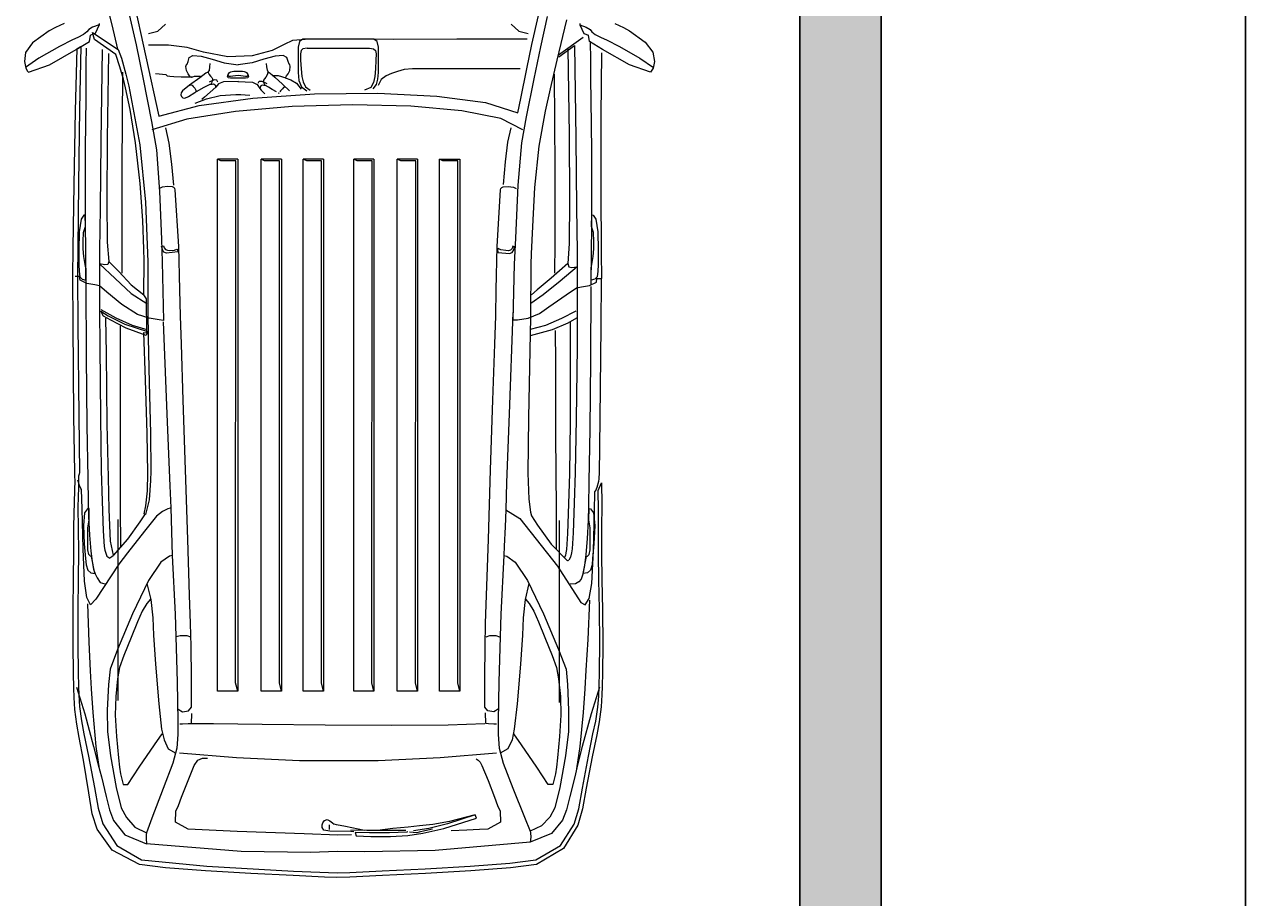
# Model space of a CAD drawing. Units: inches. Extents: x -9 to 646, y -802 to 47.
# Tile 11 of 17: x 514 to 646, y -670 to -576. Entities that reach past the tile are written whole.
import ezdxf

# ---------------------------------------------------------------- set-up
doc = ezdxf.new("R2010")
doc.units = ezdxf.units.IN
doc.header["$MEASUREMENT"] = 0
for name, color, linetype, lineweight in [('A-ANNO-DIMS', 2, 'Continuous', 18), ('A-SITE-VEHI', 8, 'Continuous', 9), ('A-WALL-PATT', 5, 'Continuous', 9), ('C-SITE', 7, 'Continuous', 25)]:
    doc.layers.add(name, color=color, linetype=linetype, lineweight=lineweight)
doc.styles.get("Standard").update_dxf_attribs({"font": 'arial.ttf'})
doc.dimstyles.get("Standard").update_dxf_attribs({"dimtxt": 0.18, "dimasz": 0.18, "dimexe": 0.18, "dimexo": 0.0625, "dimgap": 0.09, "dimtad": 0, "dimtih": 1, "dimtoh": 1, "dimdec": 0, "dimzin": 0, "dimdsep": 46, "dimlunit": 3, "dimtxsty": 'Standard', "dimcen": 0.09, "dimadec": 0, "dimazin": 0, "dimtfac": 1, "dimtdec": 0, "dimtofl": 0, "dimtmove": 0, "dimatfit": 3, "dimfxl": 1, "dimtolj": 1, "dimtzin": 0, "dimarcsym": 0})

# ---------------------------------------------------------------- blocks, each defined once
blk = doc.blocks.new('*D50')
at = {"layer": 'A-ANNO-DIMS', "color": 0, "lineweight": -2, "transparency": 16777216}
for p, q in [((606.44, 7.93), (645.8, 7.93)), ((645.62, 7.75), (645.62, -376.89)), ((645.62, -761.89), (645.62, -377.25)), ((606.44, -762.07), (645.8, -762.07))]:
    blk.add_line(p, q, dxfattribs=at)
at = {"layer": 'A-ANNO-DIMS', "color": 0, "transparency": 16777216}
for points in [[(645.59, 7.75), (645.65, 7.75), (645.62, 7.93)], [(645.59, -761.89), (645.65, -761.89), (645.62, -762.07)]]:
    blk.add_solid(points, dxfattribs=at)
at = {"layer": 'Defpoints', "color": 0, "transparency": 16777216}
for p in [(606.37, 7.93), (606.37, -762.07), (645.62, -762.07)]:
    blk.add_point(p, dxfattribs=at)
at = {"layer": 'A-ANNO-DIMS', "color": 0, "transparency": 16777216, "insert": (645.62, -377.07), "char_height": 0.18, "attachment_point": 5}
blk.add_mtext('\\A1;770', dxfattribs=at)

msp = doc.modelspace()

# ---------------------------------------------------------------- hatches: boundary and pattern name
at = {"layer": 'A-WALL-PATT'}
h = msp.add_hatch(color=256, dxfattribs=at)
h.dxf.hatch_style = 1
h.paths.add_polyline_path([(597.63, -101.57), (570.37, -101.57), (570.37, -496.07), (570.37, -511.17), (597.63, -511.17)], flags=0)
h.paths.add_polyline_path([(606.37, -101.57), (597.63, -101.57), (597.63, -511.17), (570.37, -511.17), (570.37, -513.2), (597.63, -513.2), (597.63, -712.07), (606.37, -712.07)])

# ---------------------------------------------------------------- linework, layer by layer
at = {"layer": 'A-SITE-VEHI'}
for p, q in [((525.18, -569.94), (528.59, -585.53)), ((522.94, -573.43), (523.51, -575.71)), ((518.38, -575.54), (517.46, -575.99)), ((522.17, -575.54), (522.15, -575.69)), ((525.4, -574.57), (526.13, -577.85)), ((568.77, -577.83), (569.47, -574.7)), ((570.42, -574.81), (569.69, -578.08)), ((572.5, -575.15), (571.45, -579.49)), ((573.91, -575.54), (573.92, -575.69)), ((577.69, -575.54), (578.61, -575.99)), ((516.78, -576.35), (514.99, -577.63)), ((517.46, -575.99), (516.78, -576.35)), ((520.49, -576.73), (519.85, -577.05)), ((520.85, -576.45), (520.49, -576.73)), ((521.04, -576.22), (520.85, -576.45)), ((521.45, -575.96), (521.04, -576.22)), ((521.12, -577.48), (521.23, -576.83)), ((521.72, -576.62), (521.23, -576.83)), ((522.15, -575.69), (521.45, -575.96)), ((521.46, -576.51), (524.21, -578.36)), ((521.65, -577.27), (521.46, -576.51)), ((522.15, -575.69), (521.72, -576.62)), ((523.51, -575.71), (524.15, -578.33)), ((527.46, -576.65), (528.47, -576.39)), ((528.47, -576.39), (529.3, -575.62)), ((566.53, -575.62), (567.36, -576.39)), ((567.36, -576.39), (568.37, -576.65)), ((573.92, -575.69), (574.36, -576.62)), ((573.92, -575.69), (574.62, -575.96)), ((574.36, -576.62), (574.84, -576.83)), ((574.62, -575.96), (575.03, -576.22)), ((574.95, -577.48), (574.84, -576.83)), ((575.03, -576.22), (575.22, -576.45)), ((575.22, -576.45), (575.58, -576.73)), ((575.58, -576.73), (576.22, -577.05)), ((578.61, -575.99), (579.29, -576.35)), ((579.29, -576.35), (580.96, -577.57)), ((514.99, -577.63), (514.24, -578.68)), ((517.89, -578.04), (515.68, -579.28)), ((519.28, -577.32), (517.89, -578.04)), ((519.85, -577.05), (519.28, -577.32)), ((519.69, -578.37), (521.12, -577.48)), ((519.8, -578.25), (520.2, -578.02)), ((520.2, -578.02), (520.04, -584.75)), ((523.96, -578.88), (521.65, -577.27)), ((526.13, -577.85), (526.9, -581.55)), ((529.64, -577.88), (527.47, -577.88)), ((531.63, -578.13), (529.64, -577.88)), ((533.41, -578.63), (531.63, -578.13)), ((542.07, -577.82), (540.81, -578.46)), ((543, -577.38), (542.07, -577.82)), ((544.8, -577.24), (543, -577.38)), ((543.74, -577.48), (543.6, -578.1)), ((543.6, -578.1), (543.6, -580.84)), ((544.09, -577.26), (543.74, -577.48)), ((544.58, -577.24), (544.09, -577.26)), ((551.25, -577.24), (544.58, -577.24)), ((548.41, -577.25), (544.8, -577.24)), ((553.89, -577.27), (548.41, -577.25)), ((551.74, -577.26), (551.25, -577.24)), ((552.09, -577.48), (551.74, -577.26)), ((552.23, -578.1), (552.09, -577.48)), ((552.23, -580.84), (552.23, -578.1)), ((560.68, -577.26), (553.89, -577.27)), ((568.24, -577.25), (560.68, -577.26)), ((568.21, -580.45), (568.77, -577.83)), ((569.69, -578.08), (568.97, -581.53)), ((574.3, -577.05), (571.64, -578.95)), ((571.65, -579.14), (573.35, -577.91)), ((573.35, -577.91), (573.49, -587.92)), ((576.38, -578.37), (574.95, -577.48)), ((575.04, -577.51), (575.06, -579.49)), ((576.22, -577.05), (576.8, -577.32)), ((576.8, -577.32), (578.18, -578.04)), ((578.18, -578.04), (580.39, -579.28)), ((580.96, -577.57), (581.77, -578.65)), ((514.24, -578.68), (514.12, -579.64)), ((515.68, -579.28), (514.23, -580.29)), ((516.81, -579.99), (519.69, -578.37)), ((519.62, -584.96), (519.8, -578.25)), ((520.76, -578.21), (520.74, -579.95)), ((522.5, -578.34), (522.36, -588.25)), ((523.18, -578.8), (523.04, -587.97)), ((524.4, -580.24), (523.96, -578.88)), ((524.21, -578.36), (524.58, -579.3)), ((524.58, -579.3), (525.03, -581)), ((531.73, -579.65), (531.87, -579.23)), ((531.87, -579.23), (532.25, -579.01)), ((532.25, -579.01), (533.13, -579.06)), ((533.13, -579.06), (534.33, -579.4)), ((536.02, -579.16), (533.41, -578.63)), ((534.33, -579.4), (535.61, -579.8)), ((538.63, -579.03), (536.02, -579.16)), ((540.81, -578.46), (538.63, -579.03)), ((539.91, -579.4), (538.63, -579.8)), ((541.11, -579.06), (539.91, -579.4)), ((541.98, -579.01), (541.11, -579.06)), ((542.36, -579.23), (541.98, -579.01)), ((542.5, -579.65), (542.36, -579.23)), ((543.9, -578.46), (543.84, -578.81)), ((543.84, -578.81), (543.86, -579.5)), ((543.86, -579.5), (543.91, -580.44)), ((544.11, -578.27), (543.9, -578.46)), ((544.55, -578.21), (544.11, -578.27)), ((544.55, -578.21), (551.28, -578.21)), ((551.28, -578.21), (551.72, -578.27)), ((551.72, -578.27), (551.93, -578.46)), ((551.97, -579.5), (551.92, -580.44)), ((551.93, -578.46), (551.99, -578.81)), ((551.99, -578.81), (551.97, -579.5)), ((571.45, -579.49), (570.72, -582.58)), ((572.62, -578.24), (572.76, -587.53)), ((575.06, -579.49), (575.08, -581.58)), ((576.27, -578.72), (576.19, -585.49)), ((579.26, -579.99), (576.38, -578.37)), ((580.39, -579.28), (581.85, -580.29)), ((581.77, -578.65), (581.95, -579.64)), ((514.12, -579.64), (514.25, -580.37)), ((514.25, -580.37), (514.45, -580.7)), ((514.45, -580.7), (514.55, -580.78)), ((514.55, -580.78), (516.81, -579.99)), ((520.74, -579.95), (520.74, -581.57)), ((524.77, -581.55), (524.4, -580.24)), ((524.67, -580.78), (524.6, -591.02)), ((531.5, -580.18), (531.55, -579.96)), ((531.56, -580.6), (531.5, -580.18)), ((531.55, -579.96), (531.63, -579.92)), ((531.73, -580.96), (531.56, -580.6)), ((531.63, -579.92), (531.73, -579.65)), ((533.78, -580.82), (533.64, -580.91)), ((533.83, -580.82), (533.78, -580.82)), ((533.84, -580.83), (533.83, -580.82)), ((534, -580.6), (533.84, -580.83)), ((533.9, -580.84), (534, -581.05)), ((534.06, -580.24), (534, -580.6)), ((534.08, -579.86), (534.06, -580.24)), ((535.61, -579.8), (537.12, -579.99)), ((536.19, -580.84), (536.33, -580.76)), ((536.33, -580.76), (536.48, -580.73)), ((536.48, -580.73), (536.65, -580.7)), ((536.65, -580.7), (536.88, -580.69)), ((536.88, -580.69), (537.12, -580.68)), ((538.63, -579.8), (537.12, -579.99)), ((537.12, -580.68), (537.36, -580.69)), ((537.36, -580.69), (537.58, -580.7)), ((537.58, -580.7), (537.76, -580.73)), ((537.76, -580.73), (537.9, -580.76)), ((537.9, -580.76), (538.04, -580.84)), ((540.16, -579.86), (540.18, -580.23)), ((540.18, -580.23), (540.24, -580.59)), ((540.24, -580.59), (540.4, -580.84)), ((540.34, -580.84), (540.24, -581.09)), ((540.4, -580.84), (540.41, -580.82)), ((540.41, -580.82), (540.46, -580.82)), ((540.46, -580.82), (540.59, -580.92)), ((542.61, -579.92), (542.5, -579.65)), ((542.51, -580.96), (542.68, -580.6)), ((542.69, -579.96), (542.61, -579.92)), ((542.68, -580.6), (542.74, -580.18)), ((542.74, -580.18), (542.69, -579.96)), ((543.6, -580.84), (543.68, -581.68)), ((543.91, -580.44), (544, -581.25)), ((551.92, -580.44), (551.84, -581.25)), ((552.18, -581.54), (552.23, -580.84)), ((554.28, -580.72), (553.66, -580.94)), ((555.02, -580.52), (554.28, -580.72)), ((555.89, -580.44), (555.02, -580.52)), ((567.49, -580.44), (555.89, -580.44)), ((567.56, -583.62), (568.21, -580.45)), ((581.52, -580.78), (579.26, -579.99)), ((581.62, -580.7), (581.52, -580.78)), ((581.82, -580.37), (581.62, -580.7)), ((581.95, -579.64), (581.82, -580.37)), ((520.74, -581.57), (520.71, -583.54)), ((525.01, -582.48), (524.77, -581.55)), ((525.03, -581), (525.35, -582.29)), ((526.9, -581.55), (527.79, -586.1)), ((529.38, -581.07), (528.22, -580.99)), ((529.41, -581.12), (529.38, -581.07)), ((529.53, -581.21), (529.41, -581.12)), ((529.76, -581.28), (529.53, -581.21)), ((530.2, -581.31), (529.76, -581.28)), ((531, -581.33), (530.2, -581.31)), ((532.21, -581.34), (531, -581.33)), ((531.89, -581.2), (531.73, -580.96)), ((531.99, -581.32), (531.89, -581.2)), ((532.99, -581.39), (531.9, -582.19)), ((531.94, -582.18), (532.05, -582.15)), ((532.09, -581.36), (531.99, -581.32)), ((532.05, -582.15), (532.16, -582.19)), ((532.21, -581.34), (532.09, -581.36)), ((532.38, -581.28), (532.21, -581.34)), ((532.65, -581.25), (532.38, -581.28)), ((533.09, -581.27), (532.65, -581.25)), ((533.64, -580.91), (532.99, -581.39)), ((533.41, -582.45), (534.12, -582.09)), ((534, -581.05), (534.14, -581.22)), ((534.56, -581.62), (534, -581.86)), ((534.12, -582.09), (534.13, -582.1)), ((534.13, -582.1), (534.2, -582.1)), ((534.14, -581.22), (534.28, -581.37)), ((534.2, -582.1), (534.32, -582.09)), ((534.25, -581.97), (534.23, -582.05)), ((534.23, -582.05), (534.23, -582.08)), ((534.31, -581.82), (534.25, -581.97)), ((534.28, -581.37), (534.37, -581.51)), ((534.37, -581.66), (534.31, -581.82)), ((534.32, -582.09), (534.49, -582.07)), ((534.37, -581.51), (534.37, -581.66)), ((534.49, -582.07), (534.64, -582.15)), ((534.84, -581.66), (534.56, -581.62)), ((534.64, -582.15), (534.73, -582.41)), ((535.02, -582.04), (534.73, -582.41)), ((534.95, -581.87), (534.84, -581.66)), ((535.54, -581.85), (535.02, -582.04)), ((537.16, -581.79), (535.54, -581.85)), ((535.98, -581.26), (536.06, -581.03)), ((536.05, -581.4), (535.98, -581.26)), ((536.05, -581.15), (536.06, -581.03)), ((536.13, -581.25), (536.05, -581.15)), ((536.31, -581.45), (536.05, -581.4)), ((536.06, -581.03), (536.19, -580.84)), ((536.31, -581.27), (536.13, -581.25)), ((536.56, -581.23), (536.31, -581.27)), ((537.93, -581.45), (536.31, -581.45)), ((536.85, -581.19), (536.56, -581.23)), ((537.13, -581.17), (536.85, -581.19)), ((537.08, -581.79), (538.69, -581.87)), ((537.41, -581.19), (537.13, -581.17)), ((537.68, -581.23), (537.41, -581.19)), ((537.93, -581.27), (537.68, -581.23)), ((538.1, -581.25), (537.93, -581.27)), ((538.19, -581.4), (537.93, -581.45)), ((538.04, -580.84), (538.18, -581.03)), ((538.19, -581.15), (538.1, -581.25)), ((538.18, -581.03), (538.25, -581.26)), ((538.18, -581.03), (538.19, -581.15)), ((538.25, -581.26), (538.19, -581.4)), ((538.69, -581.87), (539.19, -582.13)), ((539.19, -582.13), (539.46, -582.54)), ((539.27, -581.98), (539.39, -581.78)), ((539.39, -581.78), (539.67, -581.76)), ((539.67, -581.76), (540.22, -582.02)), ((539.87, -581.66), (539.85, -581.8)), ((539.85, -581.8), (539.91, -581.97)), ((539.96, -581.52), (539.87, -581.66)), ((539.91, -581.97), (539.96, -582.12)), ((540.1, -581.33), (539.96, -581.52)), ((539.96, -582.12), (539.98, -582.2)), ((540.24, -581.09), (540.1, -581.33)), ((540.59, -580.92), (541.07, -581.35)), ((540.95, -581.16), (541.44, -581.17)), ((541.07, -581.35), (541.9, -582.09)), ((541.44, -581.17), (541.81, -581.25)), ((541.81, -581.25), (542.03, -581.34)), ((541.9, -582.09), (542.67, -582.8)), ((542.03, -581.34), (542.15, -581.36)), ((542.15, -581.36), (542.25, -581.32)), ((542.19, -581.41), (542.8, -581.63)), ((542.25, -581.32), (542.35, -581.2)), ((542.35, -581.2), (542.51, -580.96)), ((542.8, -581.63), (543.42, -581.98)), ((543.42, -581.98), (543.92, -582.62)), ((543.68, -581.68), (543.96, -582.37)), ((544, -581.25), (544.12, -581.84)), ((544.12, -581.84), (544.38, -582.38)), ((551.7, -581.9), (551.4, -582.44)), ((551.66, -582.6), (552.01, -582.14)), ((551.84, -581.25), (551.7, -581.9)), ((552.01, -582.14), (552.18, -581.54)), ((552.52, -581.59), (552.21, -582.23)), ((553.07, -581.2), (552.52, -581.59)), ((553.66, -580.94), (553.07, -581.2)), ((568.97, -581.53), (568.16, -585.6)), ((571.16, -581.01), (571.22, -591.19)), ((575.08, -581.58), (575.11, -583.78)), ((525.49, -584.82), (525.01, -582.48)), ((525.35, -582.29), (526.54, -588.63)), ((531, -583.02), (530.96, -583.23)), ((530.96, -583.23), (531.03, -583.42)), ((531.14, -582.8), (531, -583.02)), ((531.03, -583.42), (531.16, -583.57)), ((531.9, -582.19), (531.14, -582.8)), ((531.39, -583.59), (531.77, -583.4)), ((531.77, -583.4), (532.48, -582.97)), ((532.16, -582.19), (532.3, -582.33)), ((532.3, -582.33), (532.45, -582.53)), ((532.45, -582.53), (532.57, -582.72)), ((532.48, -582.97), (533.41, -582.45)), ((532.57, -582.72), (532.59, -582.89)), ((534.12, -582.96), (533.5, -583.5)), ((533.71, -583.67), (535.21, -583.32)), ((534.73, -582.41), (534.12, -582.96)), ((535.21, -583.32), (536.88, -583.19)), ((536.88, -583.19), (537.42, -583.2)), ((537.42, -583.2), (537.9, -583.22)), ((537.9, -583.22), (538.4, -583.27)), ((538.72, -583.58), (545.36, -583.14)), ((539.57, -582.28), (539.46, -582.54)), ((539.46, -582.54), (539.62, -582.72)), ((539.72, -582.21), (539.57, -582.28)), ((539.62, -582.72), (539.79, -582.9)), ((539.88, -582.23), (539.72, -582.21)), ((539.79, -582.9), (539.99, -583.12)), ((540, -582.25), (539.88, -582.23)), ((539.98, -582.2), (539.98, -582.23)), ((540.07, -582.25), (540, -582.25)), ((540.09, -582.25), (540.07, -582.25)), ((540.39, -582.41), (540.09, -582.25)), ((540.78, -582.65), (540.39, -582.41)), ((541.25, -582.93), (540.78, -582.65)), ((541.5, -583.06), (541.47, -583.07)), ((541.47, -583.07), (541.55, -583.06)), ((541.52, -583.06), (541.5, -583.06)), ((541.55, -583.06), (541.52, -583.06)), ((541.69, -582.82), (541.61, -582.93)), ((541.78, -582.7), (541.69, -582.82)), ((541.89, -582.58), (541.78, -582.7)), ((542.03, -582.45), (541.89, -582.58)), ((542.15, -582.42), (542.03, -582.45)), ((542.25, -582.45), (542.15, -582.42)), ((543.96, -582.37), (544.53, -582.82)), ((544.38, -582.38), (544.88, -582.73)), ((545.36, -583.14), (552.17, -583.07)), ((551.4, -582.44), (550.72, -582.72)), ((552.17, -583.07), (558.52, -583.37)), ((558.52, -583.37), (563.76, -584.07)), ((570.72, -582.58), (570.18, -585.01)), ((520.04, -584.75), (519.92, -592.82)), ((520.71, -583.54), (520.64, -589.04)), ((528.59, -585.53), (532.92, -584.38)), ((531.16, -583.57), (531.39, -583.59)), ((532.49, -584.15), (533.71, -583.67)), ((532.92, -584.38), (538.72, -583.58)), ((533.5, -583.5), (533.21, -583.74)), ((542.96, -584.5), (536.83, -585.02)), ((549.44, -584.31), (542.96, -584.5)), ((555.71, -584.46), (549.44, -584.31)), ((561.22, -584.95), (555.71, -584.46)), ((563.76, -584.07), (567.24, -585.16)), ((567.24, -585.16), (567.56, -583.62)), ((575.11, -583.78), (575.18, -589.28)), ((519.47, -592.94), (519.62, -584.96)), ((526.08, -588.41), (525.49, -584.82)), ((527.79, -586.1), (528.32, -589.15)), ((531.61, -585.86), (527.83, -587.01)), ((536.83, -585.02), (531.61, -585.86)), ((565.43, -585.8), (561.22, -584.95)), ((567.77, -587.01), (565.43, -585.8)), ((568.16, -585.6), (567.64, -588.39)), ((570.18, -585.01), (569.51, -588.76)), ((576.19, -585.49), (576.2, -593.52)), ((529.29, -586.78), (529.66, -588.45)), ((566.49, -586.78), (566.15, -588.35)), ((522.36, -588.25), (522.27, -595.49)), ((523.04, -587.97), (522.99, -594.73)), ((526.58, -592.77), (526.08, -588.41)), ((526.54, -588.63), (527.14, -594.8)), ((529.66, -588.45), (529.97, -590.69)), ((566.15, -588.35), (565.88, -590.46)), ((567.64, -588.39), (567.26, -592.98)), ((572.76, -587.53), (572.82, -594.56)), ((573.49, -587.92), (573.58, -595.42)), ((520.64, -589.04), (520.64, -594.48)), ((528.32, -589.15), (528.65, -593.66)), ((569.51, -588.76), (569.04, -593.21)), ((575.18, -589.28), (575.18, -594.71)), ((524.6, -591.02), (524.6, -599.14)), ((529.97, -590.69), (530.18, -592.96)), ((534.89, -647.47), (534.89, -590.16)), ((535.26, -590.34), (534.89, -590.16)), ((537.08, -590.16), (534.89, -590.16)), ((536.88, -590.34), (535.26, -590.34)), ((536.86, -646.56), (536.88, -590.34)), ((537.08, -590.16), (537.08, -647.47)), ((537.08, -590.16), (537.08, -647.47)), ((539.6, -647.47), (539.6, -590.16)), ((539.97, -590.34), (539.6, -590.16)), ((541.79, -590.16), (539.6, -590.16)), ((541.59, -590.34), (539.97, -590.34)), ((541.57, -646.56), (541.59, -590.34)), ((541.78, -590.16), (541.78, -647.47)), ((541.79, -590.16), (541.79, -647.47)), ((544.14, -647.47), (544.14, -590.16)), ((544.51, -590.34), (544.14, -590.16)), ((546.32, -590.16), (544.14, -590.16)), ((546.12, -590.34), (544.51, -590.34)), ((546.1, -646.56), (546.12, -590.34)), ((546.32, -590.16), (546.32, -647.47)), ((546.32, -590.16), (546.32, -647.47)), ((549.57, -647.47), (549.57, -590.16)), ((549.94, -590.34), (549.57, -590.16)), ((551.75, -590.16), (549.57, -590.16)), ((551.55, -590.34), (549.94, -590.34)), ((551.53, -646.56), (551.55, -590.34)), ((551.75, -590.16), (551.75, -647.47)), ((551.75, -590.16), (551.75, -647.47)), ((554.27, -647.47), (554.27, -590.16)), ((554.64, -590.34), (554.27, -590.16)), ((556.46, -590.16), (554.27, -590.16)), ((556.26, -590.34), (554.64, -590.34)), ((556.24, -646.56), (556.26, -590.34)), ((556.46, -590.16), (556.46, -647.47)), ((556.46, -590.16), (556.46, -647.47)), ((558.81, -647.47), (558.81, -590.16)), ((559.18, -590.34), (558.81, -590.16)), ((558.81, -590.16), (561, -590.16)), ((560.8, -590.34), (559.18, -590.34)), ((560.78, -646.56), (560.8, -590.34)), ((561, -590.16), (561, -647.47)), ((565.88, -590.46), (565.68, -592.88)), ((571.22, -591.19), (571.22, -599.2)), ((519.36, -599.71), (519.47, -592.94)), ((519.92, -592.82), (519.85, -599.67)), ((526.86, -596.76), (526.58, -592.77)), ((528.65, -593.66), (528.87, -598.79)), ((528.96, -593.17), (528.66, -593.34)), ((529.54, -593.11), (528.96, -593.17)), ((530.06, -593.16), (529.54, -593.11)), ((530.19, -593.22), (530.06, -593.16)), ((530.3, -593.33), (530.19, -593.22)), ((530.34, -593.46), (530.3, -593.33)), ((530.74, -599.57), (530.34, -593.46)), ((565.01, -599.57), (565.39, -593.46)), ((565.39, -593.46), (565.43, -593.33)), ((565.43, -593.33), (565.54, -593.22)), ((565.54, -593.22), (565.67, -593.16)), ((565.67, -593.16), (566.19, -593.11)), ((566.19, -593.11), (566.77, -593.17)), ((566.77, -593.17), (567.07, -593.34)), ((567.26, -592.98), (566.98, -598.67)), ((569.04, -593.21), (568.82, -597.4)), ((576.2, -593.52), (576.23, -600.23)), ((520.64, -594.48), (520.65, -596.94)), ((522.99, -594.73), (523.03, -599.12)), ((527.14, -594.8), (527.41, -601.22)), ((572.82, -594.56), (572.79, -599.23)), ((575.18, -594.71), (575.17, -597.17)), ((520.22, -596.63), (520, -597.99)), ((520.52, -596.19), (520.22, -596.63)), ((520.67, -596.16), (520.52, -596.19)), ((520.69, -597.43), (520.67, -596.16)), ((522.27, -595.49), (522.21, -599.94)), ((573.58, -595.42), (573.62, -600.12)), ((575.19, -597.43), (575.2, -596.16)), ((575.2, -596.16), (575.35, -596.19)), ((575.35, -596.19), (575.66, -596.63)), ((575.66, -596.63), (575.87, -597.99)), ((520.49, -598.06), (520.69, -597.43)), ((520.65, -596.94), (520.71, -603.51)), ((526.98, -599.85), (526.86, -596.76)), ((568.82, -597.4), (568.7, -600.35)), ((575.17, -597.17), (575.11, -603.74)), ((575.38, -598.06), (575.19, -597.43)), ((520, -597.99), (519.97, -599.95)), ((520.44, -598.99), (520.49, -598.06)), ((520.44, -599.82), (520.44, -598.99)), ((523.03, -599.12), (523.2, -601.17)), ((524.6, -599.14), (524.61, -602.44)), ((528.87, -598.79), (528.95, -601.23)), ((566.98, -598.67), (566.87, -601.46)), ((571.22, -599.2), (571.21, -602.44)), ((572.79, -599.23), (572.62, -601.41)), ((575.43, -598.99), (575.38, -598.06)), ((575.43, -599.82), (575.43, -598.99)), ((575.87, -597.99), (575.91, -599.95)), ((519.32, -602.79), (519.36, -599.71)), ((519.85, -599.67), (519.82, -602.79)), ((519.97, -599.95), (519.99, -601.56)), ((520.51, -600.65), (520.44, -599.82)), ((522.21, -599.94), (522.19, -601.45)), ((527, -601.09), (526.98, -599.85)), ((528.89, -599.54), (529.08, -599.51)), ((528.98, -599.89), (528.89, -599.54)), ((529.14, -600.18), (528.98, -599.89)), ((529.08, -599.51), (529.16, -599.73)), ((529.43, -600.28), (529.14, -600.18)), ((529.16, -599.73), (529.31, -599.91)), ((529.31, -599.91), (529.53, -599.97)), ((530.65, -600.16), (529.43, -600.28)), ((529.53, -599.97), (529.79, -599.99)), ((529.79, -599.99), (530.27, -599.98)), ((530.27, -599.98), (530.52, -599.86)), ((530.52, -599.86), (530.62, -600)), ((530.62, -600), (530.65, -600.12)), ((530.65, -600.12), (530.65, -600.16)), ((530.86, -604.23), (530.74, -599.57)), ((564.91, -604.23), (565.01, -599.57)), ((565.13, -599.78), (565.07, -599.95)), ((565.07, -599.95), (565.1, -600.13)), ((565.1, -600.13), (565.13, -600.21)), ((565.42, -599.92), (565.13, -599.78)), ((565.13, -600.21), (566.35, -600.33)), ((565.96, -600), (565.42, -599.92)), ((566.25, -600.02), (565.96, -600)), ((566.47, -599.96), (566.25, -600.02)), ((566.35, -600.33), (566.64, -600.22)), ((566.62, -599.77), (566.47, -599.96)), ((566.7, -599.55), (566.62, -599.77)), ((566.64, -600.22), (566.8, -599.93)), ((566.89, -599.59), (566.7, -599.55)), ((566.8, -599.93), (566.89, -599.59)), ((568.7, -600.35), (568.66, -601.46)), ((573.62, -600.12), (573.63, -601.75)), ((575.36, -600.65), (575.43, -599.82)), ((575.91, -599.95), (575.89, -601.56)), ((576.23, -600.23), (576.25, -603.03)), ((519.99, -601.56), (520.01, -602.23)), ((520.64, -601.49), (520.51, -600.65)), ((520.71, -601.88), (520.64, -601.49)), ((520.71, -603.21), (520.71, -601.88)), ((522.19, -601.45), (523.9, -603.03)), ((522.78, -601.56), (522.19, -601.45)), ((522.19, -601.45), (522.21, -606.49)), ((523.08, -601.5), (522.78, -601.56)), ((523.2, -601.17), (523.08, -601.5)), ((523.2, -601.17), (524.29, -602.26)), ((526.97, -604.78), (527, -601.09)), ((527.41, -601.22), (527.39, -604.99)), ((528.95, -601.23), (529.08, -607.53)), ((566.87, -601.46), (566.71, -607.48)), ((568.66, -601.46), (568.61, -607.21)), ((572.62, -601.41), (570.82, -602.99)), ((573.63, -601.75), (571.8, -603.3)), ((572.62, -601.41), (572.74, -601.75)), ((572.74, -601.75), (573.05, -601.84)), ((573.05, -601.84), (573.63, -601.75)), ((573.63, -601.75), (573.65, -606.56)), ((575.16, -601.88), (575.23, -601.49)), ((575.16, -603.21), (575.16, -601.88)), ((575.23, -601.49), (575.36, -600.65)), ((575.89, -601.56), (575.87, -602.23)), ((519.36, -607.96), (519.32, -602.79)), ((520.06, -602.8), (519.57, -602.79)), ((519.82, -602.79), (519.86, -607.96)), ((520.01, -602.23), (520.09, -602.82)), ((520.11, -603.18), (520.06, -602.8)), ((520.09, -602.82), (520.32, -603.1)), ((520.84, -603.56), (520.11, -603.18)), ((520.32, -603.1), (520.71, -603.21)), ((523.9, -603.03), (525.62, -604.62)), ((524.29, -602.26), (525.61, -603.69)), ((570.82, -602.99), (569.34, -604.25)), ((575.55, -603.1), (575.16, -603.21)), ((575.78, -602.82), (575.55, -603.1)), ((575.71, -603.41), (575.77, -603.03)), ((575.77, -603.03), (576.23, -603.03)), ((575.87, -602.23), (575.78, -602.82)), ((576.21, -608.2), (576.25, -603.03)), ((520.71, -603.51), (520.75, -611.43)), ((521.7, -603.71), (520.84, -603.56)), ((522.21, -603.8), (521.7, -603.71)), ((523, -604.49), (522.21, -603.8)), ((524.59, -605.8), (523, -604.49)), ((525.61, -603.69), (526.97, -604.78)), ((530.91, -607.04), (530.86, -604.23)), ((564.87, -607.04), (564.91, -604.23)), ((569.34, -604.25), (568.72, -604.77)), ((571.8, -603.3), (569.99, -604.79)), ((572.47, -604.78), (573.58, -604.01)), ((573.58, -604.01), (574.1, -603.93)), ((574.1, -603.93), (574.98, -603.78)), ((574.98, -603.78), (575.71, -603.41)), ((575.12, -603.88), (575.08, -611.81)), ((526.29, -606.89), (524.59, -605.8)), ((525.62, -604.62), (527.28, -605.71)), ((527.27, -605.2), (526.97, -604.78)), ((527.29, -608.86), (527.27, -605.2)), ((527.39, -604.99), (527.41, -607.39)), ((569.99, -604.79), (568.66, -605.69)), ((570.59, -606.08), (572.47, -604.78)), ((522.21, -606.49), (522.23, -610.31)), ((522.33, -606.34), (523.96, -607.25)), ((522.63, -607.06), (522.34, -606.55)), ((522.34, -606.55), (523.14, -607.02)), ((523.41, -607.5), (522.63, -607.06)), ((523.14, -607.02), (524.91, -607.92)), ((527.53, -607.3), (526.29, -606.89)), ((531.02, -610.1), (530.91, -607.04)), ((564.76, -610.1), (564.87, -607.04)), ((566.71, -606.67), (566.3, -617.6)), ((568.36, -607.28), (569.59, -606.78)), ((569.59, -606.78), (570.59, -606.08)), ((573.5, -606.54), (571.94, -607.34)), ((573.65, -606.56), (573.62, -610.42)), ((519.45, -617.83), (519.36, -607.96)), ((519.86, -607.96), (519.96, -617.82)), ((522.86, -607.27), (522.91, -611.08)), ((525.06, -608.37), (523.41, -607.5)), ((523.96, -607.25), (525.72, -608.03)), ((524.42, -608.11), (524.43, -619.47)), ((524.91, -607.92), (527.37, -608.71)), ((527.22, -609.16), (525.06, -608.37)), ((525.72, -608.03), (527.3, -608.51)), ((527.41, -607.39), (527.42, -607.64)), ((527.42, -607.64), (527.43, -608.33)), ((527.43, -608.33), (527.45, -609.39)), ((528.62, -607.48), (527.53, -607.3)), ((529.08, -607.53), (528.62, -607.48)), ((529.06, -607.67), (529.49, -618.5)), ((566.71, -607.48), (567.21, -607.46)), ((567.21, -607.46), (568.36, -607.28)), ((568.61, -607.21), (568.54, -610.75)), ((570.21, -608.07), (568.56, -608.51)), ((571.94, -607.34), (570.21, -608.07)), ((570.98, -608.5), (572.66, -607.78)), ((572.66, -607.78), (573.6, -607.26)), ((572.87, -607.71), (572.87, -611.29)), ((576.12, -618.06), (576.21, -608.2)), ((527.14, -613.91), (526.98, -608.82)), ((526.98, -608.82), (527.29, -608.86)), ((527.37, -608.71), (527.22, -609.16)), ((527.45, -609.39), (527.56, -614.26)), ((568.61, -609.16), (570.98, -608.5)), ((571.27, -608.63), (571.29, -612.1)), ((522.23, -610.31), (522.29, -617.95)), ((522.91, -611.08), (523, -618.7)), ((531.22, -616.12), (531.02, -610.1)), ((564.56, -616.12), (564.76, -610.1)), ((568.54, -610.75), (568.41, -618.01)), ((573.62, -610.42), (573.54, -618.14)), ((520.75, -611.43), (520.84, -618.85)), ((571.29, -612.1), (571.32, -619.85)), ((572.87, -611.29), (572.87, -618.5)), ((575.08, -611.81), (574.99, -619.23)), ((527.32, -619.7), (527.14, -613.91)), ((527.56, -614.26), (527.68, -619.67)), ((531.46, -623.62), (531.22, -616.12)), ((564.32, -623.62), (564.56, -616.12)), ((566.3, -617.6), (566.04, -624.99)), ((519.53, -623.91), (519.45, -617.83)), ((519.96, -617.82), (520.04, -623.89)), ((520.84, -618.85), (520.94, -624.5)), ((522.29, -617.95), (522.39, -623.68)), ((523, -618.7), (523.12, -624.43)), ((529.49, -618.5), (529.77, -625.33)), ((568.41, -618.01), (568.33, -623.97)), ((572.87, -618.5), (572.8, -624)), ((573.54, -618.14), (573.43, -623.92)), ((576.04, -624.13), (576.12, -618.06)), ((524.43, -619.47), (524.44, -627.59)), ((527.42, -623.99), (527.32, -619.7)), ((527.68, -619.67), (527.74, -623.75)), ((571.32, -619.85), (571.36, -627.87)), ((574.99, -619.23), (574.89, -624.88)), ((519.54, -624.17), (519.53, -623.91)), ((519.55, -624.42), (519.54, -624.17)), ((519.95, -624.29), (519.94, -624.5)), ((520.01, -624.1), (519.95, -624.29)), ((520.04, -623.89), (520.01, -624.1)), ((522.39, -623.68), (522.5, -626.98)), ((527.36, -625.89), (527.42, -623.99)), ((527.74, -623.75), (527.7, -624.78)), ((531.7, -631.11), (531.46, -623.62)), ((564.08, -631.11), (564.32, -623.62)), ((568.33, -623.97), (568.43, -626.78)), ((572.8, -624), (572.69, -627.29)), ((573.43, -623.92), (573.32, -627.21)), ((576.02, -624.39), (576.04, -624.13)), ((519.49, -627.05), (519.58, -624.68)), ((519.58, -624.68), (519.55, -624.42)), ((520.04, -625.32), (519.88, -624.73)), ((519.92, -625.48), (519.88, -627.64)), ((519.94, -624.5), (519.92, -625.48)), ((520.2, -625.64), (520.04, -625.32)), ((520.94, -624.5), (520.98, -627.15)), ((523.12, -624.43), (523.2, -627.89)), ((527.7, -624.78), (527.54, -626.85)), ((529.77, -625.33), (529.87, -627.7)), ((566.04, -624.99), (565.95, -627.92)), ((574.89, -624.88), (574.85, -627.53)), ((575.63, -625.86), (575.8, -625.5)), ((575.8, -625.5), (575.97, -624.84)), ((575.89, -625.84), (576.24, -625.03)), ((575.97, -624.84), (576, -624.63)), ((576, -624.63), (576.02, -624.39)), ((576.24, -625.03), (576.29, -627.35)), ((520.27, -625.74), (520.2, -625.64)), ((520.32, -627.83), (520.27, -625.74)), ((527.54, -626.85), (527.17, -628.42)), ((527.19, -627.5), (527.36, -625.89)), ((568.43, -626.78), (568.62, -628.19)), ((575.5, -628.07), (575.55, -625.98)), ((575.55, -625.98), (575.63, -625.86)), ((575.95, -627.97), (575.89, -625.84)), ((519.44, -629.73), (519.49, -627.05)), ((519.88, -627.64), (519.9, -629.94)), ((520.44, -632.12), (520.32, -627.83)), ((520.59, -628.25), (520.46, -629.61)), ((520.9, -627.82), (520.59, -628.25)), ((521.07, -627.79), (520.9, -627.82)), ((520.98, -627.15), (521.01, -628.66)), ((521.1, -629.01), (521.07, -627.79)), ((522.5, -626.98), (522.6, -630.17)), ((523.2, -627.89), (523.33, -631.29)), ((524.44, -627.59), (524.45, -631.93)), ((527, -628.34), (527.19, -627.5)), ((528.98, -628.12), (528.35, -628.62)), ((529.55, -627.83), (528.98, -628.12)), ((529.81, -627.74), (529.55, -627.83)), ((529.87, -627.7), (530.04, -632.85)), ((565.95, -627.92), (565.87, -629.75)), ((565.95, -627.92), (567.47, -628.85)), ((568.62, -628.19), (568.71, -628.58)), ((571.36, -627.87), (571.37, -632.16)), ((572.69, -627.29), (572.59, -630.49)), ((573.32, -627.21), (573.22, -630.4)), ((574.85, -627.53), (574.82, -629.04)), ((574.89, -629.01), (574.92, -627.79)), ((574.92, -627.79), (575.09, -627.82)), ((575.09, -627.82), (575.4, -628.25)), ((575.38, -632.35), (575.5, -628.07)), ((575.4, -628.25), (575.54, -629.61)), ((575.95, -630.21), (575.95, -627.97)), ((576.29, -627.35), (576.27, -629.94)), ((520.94, -629.86), (521.1, -629.01)), ((521.01, -628.66), (521.11, -630.67)), ((524.17, -628.95), (524.17, -648.45)), ((526.55, -629.21), (525.22, -631.08)), ((527.11, -628.35), (526.55, -629.21)), ((527.17, -628.42), (527, -628.34)), ((528.35, -628.62), (527.06, -630.22)), ((567.47, -628.85), (571.53, -634)), ((568.71, -628.58), (569.36, -629.58)), ((571.69, -629.09), (571.69, -648.69)), ((574.82, -629.04), (574.72, -631.05)), ((575.05, -629.86), (574.89, -629.01)), ((519.42, -632.46), (519.44, -629.73)), ((519.9, -629.94), (519.93, -632.46)), ((520.46, -629.61), (520.56, -631.57)), ((520.94, -631.18), (520.94, -629.86)), ((521.11, -630.67), (521.25, -632.36)), ((522.6, -630.17), (522.71, -631.87)), ((527.06, -630.22), (525.22, -632.57)), ((565.87, -629.75), (565.77, -631.85)), ((569.36, -629.58), (570.85, -631.63)), ((572.59, -630.49), (572.48, -632.19)), ((573.22, -630.4), (573.11, -632.11)), ((575.05, -631.18), (575.05, -629.86)), ((575.54, -629.61), (575.44, -631.57)), ((575.93, -632.71), (575.95, -630.21)), ((576.27, -629.94), (576.25, -632.63)), ((520.6, -635.62), (520.44, -632.12)), ((520.56, -631.57), (520.69, -633.17)), ((520.96, -632.23), (520.94, -631.18)), ((522.71, -631.87), (522.78, -632.26)), ((523.33, -631.29), (523.66, -632.79)), ((525.22, -631.08), (523.67, -632.83)), ((531.89, -637.12), (531.7, -631.11)), ((563.89, -637.12), (564.08, -631.11)), ((565.77, -631.85), (565.73, -632.85)), ((570.85, -631.63), (572.51, -633.35)), ((572.48, -632.19), (572.42, -632.54)), ((573.11, -632.11), (573.02, -632.55)), ((574.72, -631.05), (574.58, -632.74)), ((575.03, -632.23), (575.05, -631.18)), ((575.44, -631.57), (575.3, -633.17)), ((519.41, -635.34), (519.42, -632.46)), ((519.93, -632.46), (519.91, -635.34)), ((520.69, -633.17), (520.76, -633.84)), ((521.06, -632.73), (520.96, -632.23)), ((521.24, -632.93), (521.06, -632.73)), ((521.34, -632.96), (521.24, -632.93)), ((521.25, -632.36), (521.41, -633.49)), ((521.7, -634.79), (521.34, -632.96)), ((521.41, -633.49), (521.57, -634.33)), ((522.78, -632.26), (522.99, -632.92)), ((522.99, -632.92), (523.31, -633.12)), ((523.31, -633.12), (523.43, -633.03)), ((523.43, -633.03), (523.54, -632.94)), ((523.54, -632.94), (523.67, -632.83)), ((525.22, -632.57), (524.29, -633.77)), ((529.72, -632.91), (528.82, -633.56)), ((530.04, -632.85), (529.72, -632.91)), ((530.04, -632.85), (530.34, -639.17)), ((565.73, -632.85), (565.43, -639.17)), ((565.73, -632.85), (566.05, -632.91)), ((566.05, -632.91), (566.95, -633.56)), ((572.37, -632.85), (572.24, -633.09)), ((572.42, -632.54), (572.37, -632.85)), ((572.51, -633.35), (572.6, -633.39)), ((572.6, -633.39), (572.68, -633.39)), ((572.68, -633.39), (572.74, -633.34)), ((572.91, -633.02), (572.74, -633.34)), ((573.02, -632.55), (572.91, -633.02)), ((574.29, -634.79), (574.65, -632.96)), ((574.58, -632.74), (574.41, -633.92)), ((574.65, -632.96), (574.75, -632.93)), ((574.75, -632.93), (574.93, -632.73)), ((574.93, -632.73), (575.03, -632.23)), ((575.22, -635.85), (575.38, -632.35)), ((575.3, -633.17), (575.24, -633.84)), ((575.97, -635.48), (575.93, -632.71)), ((576.25, -632.63), (576.29, -635.46)), ((520.76, -633.84), (520.93, -634.43)), ((520.93, -634.43), (521.25, -634.71)), ((521.25, -634.71), (521.7, -634.79)), ((521.57, -634.33), (521.74, -634.8)), ((521.74, -634.8), (521.94, -635.25)), ((524.29, -633.77), (521.81, -637.54)), ((528.82, -633.56), (527.48, -635.52)), ((566.95, -633.56), (568.29, -635.52)), ((571.53, -634), (574.04, -637.92)), ((574.41, -633.92), (574.23, -634.85)), ((574.74, -634.71), (574.29, -634.79)), ((575.07, -634.43), (574.74, -634.71)), ((575.24, -633.84), (575.07, -634.43)), ((519.38, -638.66), (519.41, -635.34)), ((519.91, -635.34), (519.88, -638.66)), ((520.83, -637.37), (520.6, -635.62)), ((521.94, -635.25), (522.27, -635.76)), ((522.27, -635.76), (522.78, -635.88)), ((527.48, -635.52), (525.76, -639.12)), ((527.31, -635.85), (527.73, -637.59)), ((568.45, -635.85), (568.04, -637.59)), ((568.29, -635.52), (570.01, -639.12)), ((573.44, -635.9), (572.87, -635.94)), ((573.83, -635.67), (573.44, -635.9)), ((574.06, -635.38), (573.83, -635.67)), ((574.23, -634.85), (574.06, -635.38)), ((574.93, -637.48), (575.22, -635.85)), ((576.04, -638.61), (575.97, -635.48)), ((576.29, -635.46), (576.36, -638.7)), ((521.23, -638.14), (520.83, -637.37)), ((532, -640.16), (531.89, -637.12)), ((563.78, -640.16), (563.89, -637.12)), ((519.37, -642.45), (519.38, -638.66)), ((519.88, -638.66), (519.87, -642.45)), ((520.89, -638.05), (521.06, -642.18)), ((521.81, -637.54), (521.23, -638.14)), ((527.29, -638.03), (526.79, -638.85)), ((527.69, -637.54), (527.29, -638.03)), ((527.73, -637.59), (527.93, -639.56)), ((568.04, -637.59), (567.83, -639.56)), ((568.07, -637.54), (568.48, -638.03)), ((568.48, -638.03), (568.98, -638.85)), ((574.04, -637.92), (574.49, -638.16)), ((574.49, -638.16), (574.93, -637.48)), ((574.97, -637.67), (574.77, -641.9)), ((576.08, -642.29), (576.04, -638.61)), ((576.36, -638.7), (576.4, -642.45)), ((525.76, -639.12), (524.14, -642.96)), ((526.28, -639.99), (525.6, -641.69)), ((526.79, -638.85), (526.28, -639.99)), ((527.93, -639.56), (528.02, -641.41)), ((530.34, -639.17), (530.56, -646.44)), ((565.43, -639.17), (565.21, -646.44)), ((567.83, -639.56), (567.75, -641.41)), ((568.98, -638.85), (569.49, -639.99)), ((569.49, -639.99), (570.17, -641.69)), ((570.01, -639.12), (571.63, -642.96)), ((528.02, -641.41), (528.22, -644.55)), ((532.07, -642.61), (532, -640.16)), ((563.72, -642.61), (563.78, -640.16)), ((567.75, -641.41), (567.54, -644.55)), ((519.39, -645.51), (519.37, -642.45)), ((519.87, -642.45), (519.9, -645.44)), ((521.06, -642.18), (521.21, -645.28)), ((525.6, -641.69), (524.82, -643.61)), ((530.47, -641.58), (530.87, -641.45)), ((530.87, -641.45), (531.6, -641.45)), ((531.6, -641.45), (531.99, -641.61)), ((532.09, -646.02), (532.07, -642.61)), ((563.69, -646.02), (563.72, -642.61)), ((564.18, -641.5), (563.79, -641.65)), ((564.91, -641.49), (564.18, -641.5)), ((565.31, -641.62), (564.91, -641.49)), ((570.17, -641.69), (570.94, -643.61)), ((574.77, -641.9), (574.58, -645.19)), ((576.05, -645.35), (576.08, -642.29)), ((576.4, -642.45), (576.37, -645.44)), ((524.14, -642.96), (523.33, -645.07)), ((524.82, -643.61), (524.37, -644.9)), ((570.94, -643.61), (571.4, -644.9)), ((571.63, -642.96), (572.44, -645.07)), ((521.21, -645.28), (521.31, -647.2)), ((523.33, -645.07), (523.16, -646.74)), ((524.37, -644.9), (524.15, -646.13)), ((528.22, -644.55), (528.58, -648.82)), ((567.54, -644.55), (567.18, -648.82)), ((571.4, -644.9), (571.61, -646.13)), ((572.44, -645.07), (572.61, -646.74)), ((574.58, -645.19), (574.46, -647.2)), ((576, -646.99), (576.05, -645.35)), ((519.44, -647.14), (519.39, -645.51)), ((519.9, -645.44), (519.95, -646.94)), ((524.15, -646.13), (523.94, -648.01)), ((530.56, -646.44), (530.64, -650.69)), ((532.1, -649.18), (532.09, -646.02)), ((537.08, -647.47), (536.86, -646.56)), ((541.78, -647.47), (541.57, -646.56)), ((546.32, -647.47), (546.1, -646.56)), ((551.75, -647.47), (551.53, -646.56)), ((556.46, -647.47), (556.24, -646.56)), ((561, -647.47), (560.78, -646.56)), ((563.69, -649.18), (563.69, -646.02)), ((565.21, -646.44), (565.13, -650.69)), ((571.61, -646.13), (571.83, -648.01)), ((576.37, -645.44), (576.32, -646.94)), ((519.46, -648.13), (519.44, -647.14)), ((519.73, -647.03), (520.63, -649.9)), ((519.95, -646.94), (519.98, -647.85)), ((519.98, -647.85), (520.06, -649.09)), ((521.31, -647.2), (521.49, -649.76)), ((523.16, -646.74), (523.04, -649.49)), ((537.08, -647.47), (534.89, -647.47)), ((541.79, -647.47), (539.6, -647.47)), ((546.32, -647.47), (544.14, -647.47)), ((551.75, -647.47), (549.57, -647.47)), ((556.46, -647.47), (554.27, -647.47)), ((561, -647.47), (558.81, -647.47)), ((572.61, -646.74), (572.72, -649.49)), ((574.46, -647.2), (574.28, -649.76)), ((576.04, -647.03), (575.14, -649.9)), ((575.87, -649.19), (575.97, -647.98)), ((575.97, -647.98), (576, -646.99)), ((576.29, -647.85), (576.21, -649.13)), ((576.32, -646.94), (576.29, -647.85)), ((519.54, -649.41), (519.46, -648.13)), ((520.06, -649.09), (520.26, -650.66)), ((523.94, -648.01), (523.87, -650.03)), ((528.58, -648.82), (528.89, -651.56)), ((531.77, -649.58), (532.1, -649.18)), ((564.01, -649.58), (563.69, -649.18)), ((567.18, -648.82), (566.87, -651.56)), ((571.83, -648.01), (571.89, -650.03)), ((575.63, -650.69), (575.87, -649.19)), ((576.21, -649.13), (576.01, -650.74)), ((519.75, -651.02), (519.54, -649.41)), ((520.63, -649.9), (521.57, -653.42)), ((521.49, -649.76), (521.82, -653.4)), ((523.04, -649.49), (523.06, -651.78)), ((523.87, -650.03), (524.03, -652.34)), ((530.66, -649.38), (531.13, -649.67)), ((531.13, -649.67), (531.77, -649.58)), ((532.1, -649.84), (532.06, -650.96)), ((563.72, -649.8), (563.75, -650.91)), ((564.65, -649.67), (564.01, -649.58)), ((565.12, -649.38), (564.65, -649.67)), ((571.89, -650.03), (571.74, -652.34)), ((572.72, -649.49), (572.71, -651.78)), ((574.28, -649.76), (573.94, -653.4)), ((575.14, -649.9), (574.19, -653.42)), ((520.01, -652.44), (519.75, -651.02)), ((520.26, -650.66), (520.52, -652.05)), ((523.06, -651.78), (523.4, -654.4)), ((528.89, -651.56), (529.15, -652.7)), ((530.64, -650.69), (530.64, -652.11)), ((531.15, -651), (530.86, -651.02)), ((531.74, -650.98), (531.15, -651)), ((532.06, -650.96), (531.74, -650.98)), ((534.48, -650.97), (532.06, -650.96)), ((539.71, -651.03), (534.48, -650.97)), ((546.5, -651.1), (539.71, -651.03)), ((553.6, -651.14), (546.5, -651.1)), ((559.75, -651.11), (553.6, -651.14)), ((563.71, -650.96), (559.75, -651.11)), ((563.75, -650.91), (564.08, -650.93)), ((564.08, -650.93), (564.67, -650.96)), ((564.67, -650.96), (564.96, -650.97)), ((565.13, -650.69), (565.12, -652.11)), ((566.87, -651.56), (566.62, -652.7)), ((572.71, -651.78), (572.37, -654.4)), ((575.34, -652.04), (575.63, -650.69)), ((576.01, -650.74), (575.74, -652.17)), ((520.47, -654.89), (520.01, -652.44)), ((520.52, -652.05), (521.01, -654.44)), ((524.03, -652.34), (524.25, -654.62)), ((526.47, -655.63), (528.12, -653.24)), ((528.12, -653.24), (528.95, -652.05)), ((529.15, -652.7), (529.59, -653.68)), ((530.64, -652.11), (530.53, -653.58)), ((565.12, -652.11), (565.24, -653.58)), ((566.62, -652.7), (566.18, -653.68)), ((567.65, -653.24), (566.82, -652.05)), ((569.3, -655.63), (567.65, -653.24)), ((571.74, -652.34), (571.52, -654.62)), ((574.85, -654.45), (575.34, -652.04)), ((575.74, -652.17), (575.25, -654.54)), ((521.01, -654.44), (521.67, -657.84)), ((521.57, -653.42), (522.07, -655.38)), ((521.82, -653.4), (522.18, -655.82)), ((523.4, -654.4), (524, -657.83)), ((529.59, -653.68), (530.42, -654.13)), ((530.53, -653.58), (530.1, -655.22)), ((536.95, -654.64), (530.8, -654.13)), ((564.96, -654.13), (558.88, -654.64)), ((565.24, -653.58), (565.67, -655.22)), ((566.18, -653.68), (565.34, -654.13)), ((572.37, -654.4), (571.76, -657.83)), ((573.94, -653.4), (573.58, -655.82)), ((574.19, -653.42), (573.69, -655.38)), ((574.2, -657.9), (574.85, -654.45)), ((575.25, -654.54), (574.6, -657.91)), ((521.05, -658.4), (520.47, -654.89)), ((522.07, -655.38), (522.4, -656.69)), ((524.25, -654.62), (524.37, -655.65)), ((524.37, -655.65), (524.46, -656.37)), ((525.24, -657.51), (526.47, -655.63)), ((530.1, -655.22), (529.07, -657.93)), ((531.73, -657.06), (532.39, -655.44)), ((532.39, -655.44), (532.78, -654.89)), ((532.78, -654.89), (533.28, -654.68)), ((533.28, -654.68), (533.83, -654.67)), ((543.74, -654.94), (536.95, -654.64)), ((547.99, -654.94), (543.74, -654.94)), ((552.19, -654.94), (547.99, -654.94)), ((558.88, -654.64), (552.19, -654.94)), ((562.75, -654.75), (562.99, -654.89)), ((562.99, -654.89), (563.2, -655.11)), ((563.2, -655.11), (563.38, -655.44)), ((563.38, -655.44), (564.04, -657.06)), ((565.67, -655.22), (566.72, -657.89)), ((570.53, -657.51), (569.3, -655.63)), ((571.4, -655.65), (571.31, -656.37)), ((571.52, -654.62), (571.4, -655.65)), ((573.69, -655.38), (573.37, -656.69)), ((522.4, -656.69), (522.91, -658.78)), ((524.46, -656.37), (524.75, -657.49)), ((531.02, -658.88), (531.73, -657.06)), ((564.04, -657.06), (564.74, -658.88)), ((571.31, -656.37), (571.02, -657.49)), ((573.37, -656.69), (572.85, -658.78)), ((521.4, -660.67), (521.05, -658.4)), ((521.67, -657.84), (522.05, -660.04)), ((524, -657.83), (524.53, -660.02)), ((524.75, -657.49), (525.24, -657.51)), ((529.07, -657.93), (527.85, -661.14)), ((566.72, -657.89), (567.97, -661.01)), ((571.02, -657.49), (570.53, -657.51)), ((571.76, -657.83), (571.24, -660.02)), ((573.81, -660.13), (574.2, -657.9)), ((574.6, -657.91), (574.22, -660.11)), ((522.91, -658.78), (523.27, -660.24)), ((530.42, -660.37), (530.7, -659.75)), ((530.7, -659.75), (531.02, -658.88)), ((564.74, -658.88), (565.07, -659.75)), ((565.07, -659.75), (565.35, -660.37)), ((572.85, -658.78), (572.49, -660.24)), ((521.94, -662.3), (521.4, -660.67)), ((522.05, -660.04), (522.56, -661.73)), ((523.27, -660.24), (523.72, -661.39)), ((524.53, -660.02), (525.09, -661.05)), ((525.09, -661.05), (526, -662.09)), ((527.85, -661.14), (527.26, -662.69)), ((530.37, -661.57), (530.42, -660.37)), ((559.28, -662.25), (562.78, -661.14)), ((562.67, -660.78), (559.66, -661.75)), ((562.67, -660.78), (559.9, -661.47)), ((562.78, -661.14), (562.67, -660.78)), ((565.35, -660.37), (565.39, -661.57)), ((567.97, -661.01), (568.58, -662.52)), ((570.69, -661.01), (569.81, -661.97)), ((571.24, -660.02), (570.69, -661.01)), ((572.49, -660.24), (572.06, -661.35)), ((573.31, -661.78), (573.81, -660.13)), ((574.22, -660.11), (573.71, -661.88)), ((523.55, -664.56), (521.94, -662.3)), ((522.56, -661.73), (524.05, -664.08)), ((523.72, -661.39), (524.94, -662.92)), ((526, -662.09), (527.26, -662.69)), ((531.73, -662.31), (530.37, -661.57)), ((537.01, -662.55), (531.73, -662.31)), ((546.18, -661.83), (546.24, -661.62)), ((546.19, -662.15), (546.18, -661.83)), ((546.34, -662.43), (546.19, -662.15)), ((546.24, -661.62), (546.44, -661.37)), ((546.99, -662.53), (546.34, -662.43)), ((546.44, -661.37), (546.71, -661.26)), ((546.71, -661.26), (547.01, -661.4)), ((546.95, -662.35), (546.98, -661.86)), ((547.01, -661.4), (547.28, -661.64)), ((547.28, -661.64), (547.48, -661.79)), ((547.72, -661.84), (547.48, -661.79)), ((548.69, -662.02), (547.72, -661.84)), ((550.74, -662.44), (548.69, -662.02)), ((550.97, -662.44), (549.26, -662.43)), ((553.74, -662.44), (550.97, -662.44)), ((553.78, -662.24), (552.12, -662.44)), ((555.19, -662.45), (553.74, -662.44)), ((555.43, -662.09), (553.78, -662.24)), ((556.65, -661.97), (555.43, -662.09)), ((557.66, -662.23), (556.01, -662.51)), ((558.11, -661.8), (556.65, -661.97)), ((557.02, -662.76), (559.28, -662.25)), ((558.05, -662.33), (557.25, -662.51)), ((559.66, -661.75), (557.66, -662.23)), ((559.9, -661.47), (558.11, -661.8)), ((561.76, -662.43), (560.07, -662.5)), ((563.11, -662.36), (561.76, -662.43)), ((564.03, -662.31), (563.11, -662.36)), ((565.39, -661.57), (564.03, -662.31)), ((569.81, -661.97), (568.58, -662.52)), ((572.06, -661.35), (570.87, -662.79)), ((571.84, -664.08), (573.31, -661.78)), ((573.71, -661.88), (572.18, -664.41)), ((524.94, -662.92), (527.26, -663.89)), ((527.23, -662.88), (527.21, -663.33)), ((527.21, -663.33), (527.26, -663.89)), ((527.26, -662.69), (527.23, -662.88)), ((544.24, -662.83), (537.01, -662.55)), ((547.88, -662.97), (544.24, -662.83)), ((549.28, -662.58), (546.99, -662.53)), ((549.34, -662.91), (547.88, -662.97)), ((549.6, -662.59), (549.28, -662.58)), ((551.29, -662.72), (549.74, -662.68)), ((549.74, -662.68), (549.85, -663.04)), ((549.85, -663.04), (551.4, -663.09)), ((553.42, -662.72), (551.29, -662.72)), ((551.4, -663.09), (553.53, -663.09)), ((555.3, -662.62), (553.42, -662.72)), ((553.53, -663.09), (555.41, -662.98)), ((555.32, -662.62), (555.3, -662.62)), ((555.34, -662.61), (555.32, -662.62)), ((555.37, -662.61), (555.34, -662.61)), ((555.41, -662.98), (557.02, -662.76)), ((556.38, -662.69), (555.58, -662.63)), ((556.63, -662.64), (556.38, -662.69)), ((557.25, -662.51), (556.63, -662.64)), ((568.58, -663.72), (558.33, -664.61)), ((568.58, -662.52), (568.6, -662.71)), ((570.87, -662.79), (568.58, -663.72)), ((568.63, -663.16), (568.58, -663.72)), ((568.6, -662.71), (568.63, -663.16)), ((526.5, -666.1), (523.55, -664.56)), ((524.05, -664.08), (526.73, -665.63)), ((537.47, -664.73), (527.26, -663.89)), ((544.93, -664.81), (537.47, -664.73)), ((547.83, -664.71), (544.93, -664.81)), ((550.77, -664.77), (547.83, -664.71)), ((558.33, -664.61), (550.77, -664.77)), ((569.17, -665.61), (571.84, -664.08)), ((572.18, -664.41), (569.27, -666.1)), ((529.31, -666.46), (526.5, -666.1)), ((526.73, -665.63), (533.75, -666.3)), ((533.75, -666.3), (543.1, -666.82)), ((557.26, -666.58), (562.11, -666.29)), ((562.11, -666.29), (566.37, -665.96)), ((566.37, -665.96), (569.17, -665.61)), ((569.27, -666.1), (566.46, -666.46)), ((533.6, -666.79), (529.31, -666.46)), ((538.48, -667.08), (533.6, -666.79)), ((543.05, -667.32), (538.48, -667.08)), ((546.44, -667.47), (543.05, -667.32)), ((543.1, -666.82), (547.78, -667.02)), ((547.76, -667.53), (546.44, -667.47)), ((549.15, -667.47), (547.76, -667.53)), ((547.78, -667.02), (549.16, -666.97)), ((552.66, -667.32), (549.15, -667.47)), ((549.16, -666.97), (552.64, -666.81)), ((552.64, -666.81), (557.26, -666.58)), ((557.29, -667.08), (552.66, -667.32)), ((562.17, -666.79), (557.29, -667.08)), ((566.46, -666.46), (562.17, -666.79))]:
    msp.add_line(p, q, dxfattribs=at)
at = {"layer": 'C-SITE'}
for p, q in [((606.37, -101.57), (606.37, -762.07)), ((597.63, -513.2), (597.63, -762.07))]:
    msp.add_line(p, q, dxfattribs=at)

# ---------------------------------------------------------------- dimensions: what is measured, and where the dimension line sits
at = {"layer": 'A-ANNO-DIMS'}
dim = msp.add_linear_dim(base=(645.62, -762.07), p1=(606.37, 7.93), p2=(606.37, -762.07), angle=90, dimstyle='Standard', override={"dimdec": 0, "dimlfac": 1, "dimrnd": 0, "dimzin": 0, "dimdsep": 46, "dimlunit": 2}, dxfattribs=at)
dim.commit()
dim.dimension.update_dxf_attribs({"geometry": '*D50', "text_midpoint": (645.62, -377.07)})

doc.saveas('drawing.dxf')
